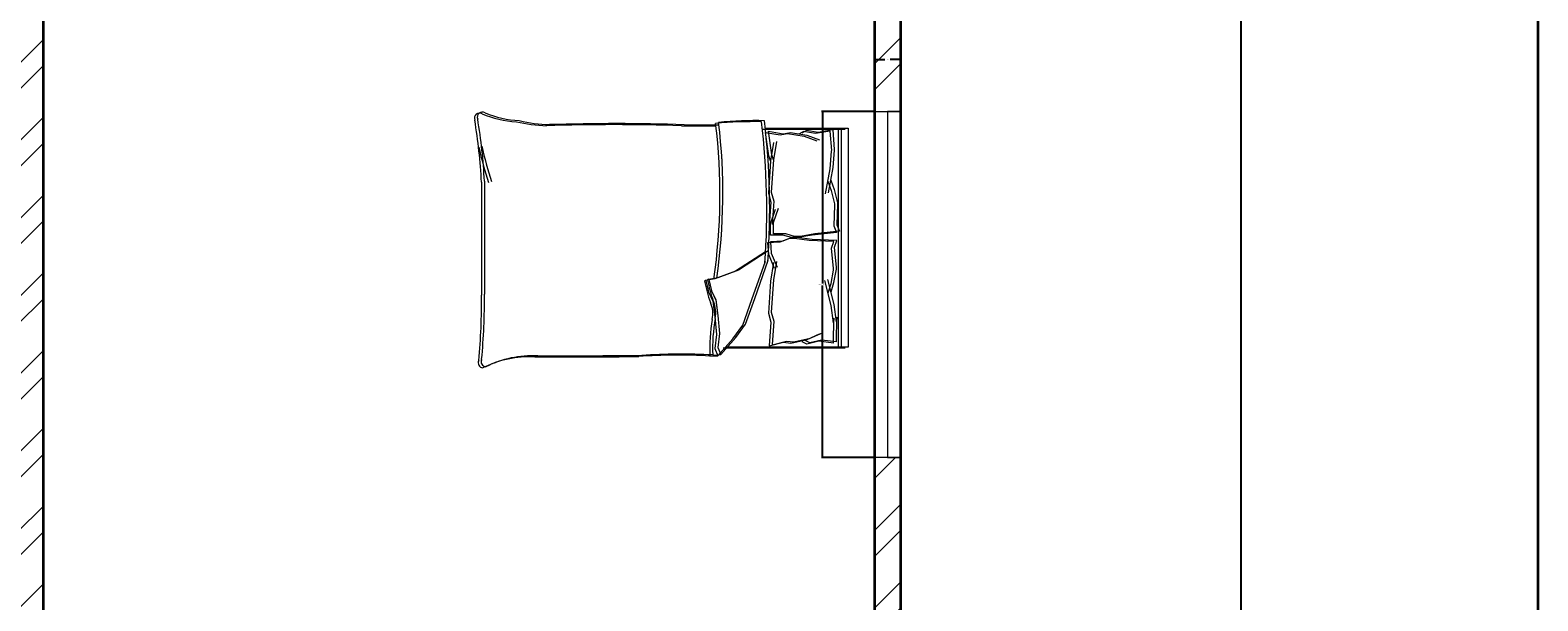
# Model space of a CAD drawing. Units: inches. Extents: x 1962 to 2771, y 1245 to 2660.
# Tile 113 of 114: x 2510 to 2771, y 2348 to 2447. Entities that reach past the tile are written whole.
import ezdxf

# ---------------------------------------------------------------- set-up
doc = ezdxf.new("R2010")
doc.units = ezdxf.units.IN
for name, color, linetype, lineweight in [('A-ANNO-DIMS', 2, 'Continuous', 18), ('A-ANNO-TTLB', 7, 'Continuous', 35), ('A-FURN', 8, 'Continuous', 13), ('A-GLAZ', 4, 'Continuous', 18), ('A-WALL', 7, 'Continuous', 35), ('A-WALL-PATT', 252, 'Continuous', 13)]:
    doc.layers.add(name, color=color, linetype=linetype, lineweight=lineweight)
doc.styles.get("Standard").update_dxf_attribs({"font": 'arial.ttf'})
doc.dimstyles.get("Standard").update_dxf_attribs({"dimtxt": 0.18, "dimasz": 0.18, "dimexe": 0.18, "dimexo": 0.0625, "dimgap": 0.09, "dimtad": 0, "dimtih": 1, "dimtoh": 1, "dimdec": 4, "dimzin": 0, "dimdsep": 46, "dimtxsty": 'Standard', "dimcen": 0.09, "dimadec": 0, "dimazin": 0, "dimtfac": 1, "dimtdec": 4, "dimtofl": 0, "dimtmove": 0, "dimatfit": 3, "dimfxl": 1, "dimtolj": 1, "dimtzin": 0, "dimarcsym": 0})

# ---------------------------------------------------------------- blocks, each defined once
blk = doc.blocks.new('BED-PLAN')
for p, q in [((22.05, 42.03), (19.47, 39.08)), ((22.05, 42.02), (19.47, 39.08)), ((22.56, 42.21), (19.98, 39.26)), ((22.56, 42.21), (19.98, 39.26)), ((23.44, 42.09), (22.05, 42.03, 3.08)), ((23.44, 42.09), (22.05, 42.02, 3.08)), ((22.55, 40.8), (22.05, 42.03)), ((22.55, 40.8), (22.05, 42.02)), ((23.95, 42.27), (22.56, 42.21, 3.08)), ((23.95, 42.27), (22.56, 42.21, 3.08)), ((23.06, 40.98), (22.56, 42.21)), ((23.06, 40.98), (22.56, 42.21)), ((0, 40.75), (21.15, 40.75)), ((0, 40.75), (21.15, 40.75)), ((0, 2.76), (0, 40.75)), ((0.51, 40.93), (21.66, 40.93)), ((0.51, 40.93), (21.66, 40.93)), ((1.22, 2.76), (1.22, 40.75)), ((1.22, 2.76), (1.22, 40.75)), ((1.73, 2.95), (1.73, 40.93)), ((1.73, 2.95), (1.73, 40.93)), ((2.03, 39.83), (1.96, 35.54)), ((2.03, 39.83), (1.96, 35.54)), ((2.03, 39.83), (4.58, 39.53)), ((2.03, 39.83), (4.58, 39.53)), ((2.54, 40.02), (2.46, 35.72)), ((2.54, 40.02), (2.46, 35.72)), ((2.54, 40.02), (5.09, 39.72)), ((2.54, 40.02), (5.09, 39.72)), ((6.56, 39.2), (4.43, 38.26)), ((6.56, 39.2), (4.43, 38.26)), ((4.58, 39.53), (6.63, 40.01)), ((4.58, 39.53), (6.63, 40.01)), ((7.07, 39.38), (4.94, 38.44)), ((7.07, 39.38), (4.94, 38.44)), ((5.09, 39.72), (7.14, 40.19)), ((5.09, 39.72), (7.14, 40.19)), ((9.4, 39.83), (6.56, 39.2)), ((9.4, 39.83), (6.56, 39.2)), ((6.63, 40.01), (7.46, 39.6)), ((6.63, 40.01), (7.46, 39.6)), ((9.91, 40.02), (7.07, 39.38)), ((9.91, 40.02), (7.07, 39.38)), ((7.14, 40.19), (7.97, 39.78)), ((7.14, 40.19), (7.97, 39.78)), ((10.68, 39.68), (9.4, 39.83)), ((10.68, 39.68), (9.4, 39.83)), ((11.19, 39.87), (9.91, 40.02)), ((11.19, 39.87), (9.91, 40.02)), ((13.17, 40.3), (10.68, 39.68)), ((13.17, 40.3), (10.68, 39.68)), ((13.68, 40.48), (11.19, 39.87)), ((13.68, 40.48), (11.19, 39.87)), ((12.85, 36.22), (13.17, 40.3)), ((12.85, 36.22), (13.17, 40.3)), ((13.36, 36.4), (13.68, 40.48)), ((13.36, 36.4), (13.68, 40.48)), ((19.98, 39.26), (18.26, 36.92)), ((19.98, 39.26), (18.26, 36.92)), ((22.3, 38.34), (22.55, 40.8)), ((22.3, 38.34), (22.55, 40.8)), ((22.81, 38.52), (23.06, 40.98)), ((22.81, 38.52), (23.06, 40.98)), ((17.75, 36.74), (16.15, 32.31)), ((17.75, 36.74), (16.15, 32.31)), ((18.26, 36.92), (16.66, 32.49)), ((18.26, 36.92), (16.66, 32.49)), ((19.47, 39.08), (17.75, 36.74)), ((19.47, 39.08), (17.75, 36.74)), ((22.55, 35.26), (22.3, 38.34)), ((22.55, 35.26), (22.3, 38.34)), ((23.06, 35.45), (22.81, 38.52)), ((23.06, 35.44), (22.81, 38.52)), ((1.96, 35.54), (2.02, 36.34)), ((1.96, 35.54), (2.02, 36.34)), ((2.02, 36.34), (2.44, 33.32)), ((2.02, 36.34), (2.44, 33.32)), ((2.46, 35.72), (2.53, 36.52)), ((2.46, 35.72), (2.53, 36.52)), ((2.53, 36.52), (2.95, 33.5)), ((2.53, 36.52), (2.95, 33.5)), ((13.3, 34.66), (12.85, 36.22)), ((13.3, 34.66), (12.85, 36.22)), ((12.95, 29.09), (13.3, 34.66)), ((12.95, 29.09), (13.3, 34.66)), ((13.8, 34.84), (13.36, 36.4)), ((13.8, 34.84), (13.36, 36.4)), ((13.46, 29.27), (13.8, 34.84)), ((13.46, 29.27), (13.8, 34.84)), ((22.92, 32.56), (22.55, 35.26)), ((22.92, 32.55), (22.55, 35.26)), ((23.42, 32.74), (23.06, 35.45)), ((23.42, 32.74), (23.06, 35.44)), ((2.44, 33.32), (3.52, 29.01)), ((2.44, 33.32), (3.52, 29.01)), ((2.95, 33.5), (4.02, 29.19)), ((2.95, 33.5), (4.02, 29.19)), ((3.43, 31.34), (2.96, 29.7)), ((3.43, 31.34), (2.96, 29.7)), ((16.15, 32.31), (13.82, 25.68)), ((16.15, 32.31), (13.82, 25.68)), ((16.66, 32.49), (14.33, 25.86)), ((16.66, 32.49), (14.33, 25.86)), ((23.65, 30.95), (22.92, 32.56)), ((23.65, 30.95), (22.92, 32.55)), ((24.16, 31.14), (23.42, 32.74)), ((24.16, 31.14), (23.42, 32.74)), ((62.99, 11.98), (62.99, 31.54)), ((62.99, 11.97), (62.99, 31.54)), ((63.5, 12.16), (63.5, 31.72)), ((63.5, 12.16), (63.5, 31.72)), ((2.45, 29.52), (2.02, 27.19)), ((2.45, 29.52), (2.02, 27.19)), ((2.92, 31.16), (2.45, 29.52)), ((2.92, 31.16), (2.45, 29.52)), ((2.96, 29.7), (2.52, 27.37)), ((2.96, 29.7), (2.52, 27.37)), ((12.42, 25.89), (12.95, 29.09)), ((12.42, 25.89), (12.95, 29.09)), ((12.93, 26.07), (13.46, 29.27)), ((12.93, 26.07), (13.46, 29.27)), ((18.98, 27.38), (22.55, 28.74)), ((18.98, 27.38), (22.55, 28.74)), ((19.49, 27.57), (23.06, 28.92)), ((19.49, 27.57), (23.06, 28.92)), ((22.55, 28.74), (24.15, 28.99)), ((22.55, 28.74), (24.15, 28.98)), ((23.06, 28.92), (24.65, 29.17)), ((23.06, 28.92), (24.65, 29.17)), ((24.15, 28.99), (23.65, 30.95)), ((24.15, 28.98), (23.65, 30.95)), ((24.65, 29.17), (24.16, 31.14)), ((24.65, 29.17), (24.16, 31.14)), ((2.02, 27.19), (2.03, 26.94)), ((2.02, 27.19), (2.03, 26.93)), ((2.03, 26.94), (2.37, 23.42)), ((2.03, 26.93), (2.37, 23.42)), ((2.52, 27.37), (2.54, 27.12)), ((2.52, 27.37), (2.54, 27.12)), ((2.54, 27.12), (2.88, 23.6)), ((2.54, 27.12), (2.88, 23.6)), ((13.31, 24.44), (12.28, 26.89)), ((13.31, 24.44), (12.28, 26.88)), ((13.81, 24.63), (12.79, 27.07)), ((13.81, 24.63), (12.79, 27.07)), ((13.82, 24.05), (18.98, 27.38)), ((13.82, 24.05), (18.98, 27.38)), ((14.33, 24.24), (19.49, 27.57)), ((14.33, 24.24), (19.49, 27.57)), ((2.88, 23.6), (2.49, 22.42)), ((2.88, 23.6), (2.49, 22.42)), ((13.43, 22.49), (13.31, 24.44)), ((13.43, 22.49), (13.31, 24.44)), ((13.94, 22.68), (13.81, 24.63)), ((13.94, 22.68), (13.81, 24.63)), ((1.49, 20.65), (5.74, 21.11)), ((1.49, 20.65), (5.74, 21.11)), ((2.37, 23.42), (1.98, 22.24)), ((2.37, 23.42), (1.98, 22.24)), ((1.98, 22.24), (6.25, 22.05)), ((1.98, 22.24), (6.25, 22.05)), ((1.99, 20.84), (6.25, 21.3)), ((1.99, 20.84), (6.25, 21.3)), ((2.49, 22.42), (6.76, 22.23)), ((2.49, 22.42), (6.76, 22.23)), ((5.74, 21.11), (8.27, 21.57)), ((5.74, 21.11), (8.27, 21.57)), ((6.25, 22.05), (8.81, 21.75)), ((6.25, 22.05), (8.81, 21.75)), ((6.25, 21.3), (8.78, 21.76)), ((6.25, 21.3), (8.78, 21.76)), ((6.76, 22.23), (9.31, 21.93)), ((6.76, 22.23), (9.31, 21.93)), ((8.27, 21.57), (9.3, 21.57)), ((8.27, 21.57), (9.3, 21.57)), ((8.78, 21.76), (9.81, 21.76)), ((8.78, 21.76), (9.81, 21.76)), ((8.81, 21.75), (9.84, 21.81)), ((8.81, 21.75), (9.84, 21.81)), ((9.3, 21.57), (10.8, 21.11)), ((9.3, 21.57), (10.8, 21.11)), ((9.31, 21.93), (10.35, 21.99)), ((9.31, 21.93), (10.35, 21.99)), ((9.81, 21.76), (11.3, 21.3)), ((9.81, 21.76), (11.3, 21.3)), ((9.84, 21.81), (11.3, 22.36)), ((9.84, 21.81), (11.3, 22.36)), ((10.35, 21.99), (11.81, 22.54)), ((10.35, 21.99), (11.81, 22.54)), ((10.8, 21.11), (12.93, 21.11)), ((10.8, 21.11), (12.93, 21.11)), ((11.3, 22.36), (13.43, 22.49)), ((11.3, 22.36), (13.43, 22.49)), ((11.3, 21.3), (13.44, 21.3)), ((11.3, 21.3), (13.44, 21.3)), ((11.81, 22.54), (13.94, 22.68)), ((11.81, 22.54), (13.94, 22.68)), ((12.93, 21.11), (12.93, 19.16)), ((12.93, 21.11), (12.93, 19.16)), ((13.44, 21.3), (13.44, 19.34)), ((13.44, 21.3), (13.44, 19.34)), ((1.95, 19.51), (1.49, 20.65)), ((1.95, 19.51), (1.49, 20.65)), ((1.83, 15.97), (1.95, 19.51)), ((1.83, 15.97), (1.95, 19.51)), ((2.45, 19.69), (1.99, 20.84)), ((2.45, 19.69), (1.99, 20.84)), ((2.34, 16.15), (2.45, 19.69)), ((2.34, 16.15), (2.45, 19.69)), ((12.93, 19.16), (12.06, 16.66)), ((12.93, 19.16), (12.06, 16.66)), ((13.44, 19.34), (12.57, 16.84)), ((13.44, 19.34), (12.57, 16.84)), ((12.85, 15.41), (13.17, 19.49)), ((12.85, 15.41), (13.17, 19.49)), ((13.36, 15.59), (13.68, 19.67)), ((13.36, 15.59), (13.68, 19.67)), ((1.83, 15.72), (1.83, 15.97)), ((1.83, 15.72), (1.83, 15.97)), ((2.41, 13.42), (1.83, 15.72)), ((2.41, 13.42), (1.83, 15.72)), ((2.34, 15.9), (2.34, 16.15)), ((2.34, 15.9), (2.34, 16.15)), ((2.91, 13.6), (2.34, 15.9)), ((2.91, 13.6), (2.34, 15.9)), ((2.98, 11.81), (2.41, 13.42)), ((2.98, 11.81), (2.41, 13.42)), ((2.64, 9.63), (3.44, 13.99)), ((2.64, 9.63), (3.44, 13.99)), ((3.49, 11.99), (2.91, 13.6)), ((3.49, 11.99), (2.91, 13.6)), ((3.14, 9.81), (3.95, 14.17)), ((3.14, 9.81), (3.95, 14.17)), ((13.3, 13.85), (12.85, 15.41)), ((13.3, 13.85), (12.85, 15.41)), ((12.95, 8.28), (13.3, 13.85)), ((12.95, 8.28), (13.3, 13.85)), ((13.8, 14.03), (13.36, 15.59)), ((13.8, 14.03), (13.36, 15.59)), ((13.46, 8.46), (13.8, 14.03)), ((13.46, 8.46), (13.8, 14.03)), ((2.41, 6.59), (2.64, 9.63)), ((2.41, 6.59), (2.64, 9.63)), ((2.91, 6.77), (3.14, 9.81)), ((2.91, 6.77), (3.14, 9.81)), ((12.42, 5.07), (12.95, 8.28)), ((12.42, 5.07), (12.95, 8.28)), ((12.93, 5.26), (13.46, 8.46)), ((12.93, 5.26), (13.46, 8.46)), ((12.95, 8.28), (13.21, 7.38)), ((12.95, 8.28), (13.21, 7.38)), ((13.46, 8.46), (13.72, 7.56)), ((13.46, 8.46), (13.72, 7.56)), ((2.39, 6.5), (2.41, 6.59)), ((2.39, 6.5), (2.41, 6.59)), ((2.65, 3.1), (2.39, 6.5)), ((2.65, 3.1), (2.39, 6.5)), ((2.9, 6.68), (2.91, 6.77)), ((2.9, 6.68), (2.91, 6.77)), ((3.16, 3.28), (2.9, 6.68)), ((3.16, 3.28), (2.9, 6.68)), ((13.21, 7.38), (13.78, 3.33)), ((13.21, 7.38), (13.78, 3.33)), ((13.72, 7.56), (14.29, 3.51)), ((13.72, 7.56), (14.29, 3.51)), ((14.4, 2.76), (0, 2.76)), ((14.4, 2.76), (0, 2.76)), ((14.9, 2.95), (0.51, 2.95)), ((14.9, 2.95), (0.51, 2.95)), ((2.64, 3.1), (5.16, 3.56)), ((2.64, 3.1), (5.16, 3.56)), ((3.14, 3.28), (5.67, 3.74)), ((3.14, 3.28), (5.67, 3.74)), ((7.12, 4.02), (4.93, 4.82)), ((7.12, 4.02), (4.93, 4.82)), ((5.16, 3.56), (7.23, 3.21)), ((5.16, 3.56), (7.23, 3.21)), ((7.63, 4.2), (5.44, 5)), ((7.63, 4.2), (5.44, 5)), ((5.67, 3.74), (7.74, 3.39)), ((5.67, 3.74), (7.74, 3.39)), ((9.99, 3.56), (7.12, 4.02)), ((9.99, 3.56), (7.12, 4.02)), ((7.23, 3.21), (8.04, 3.67)), ((7.23, 3.21), (8.04, 3.67)), ((10.5, 3.74), (7.63, 4.2)), ((10.5, 3.74), (7.63, 4.2)), ((7.74, 3.39), (8.55, 3.85)), ((7.74, 3.39), (8.55, 3.85)), ((11.26, 3.79), (9.99, 3.56)), ((11.26, 3.79), (9.99, 3.56)), ((11.76, 3.97), (10.5, 3.74)), ((11.76, 3.97), (10.5, 3.74)), ((13.78, 3.33), (11.26, 3.79)), ((13.78, 3.33), (11.26, 3.79)), ((14.29, 3.51), (11.76, 3.97)), ((14.29, 3.51), (11.76, 3.97))]:
    blk.add_line(p, q)
for centre, radius, start, end in [((-5.29, 40.8), 28.76, 349.8763, 2.5657), ((-5.29, 40.8), 28.76, 349.8763, 2.5657), ((28.87, 144.88), 102.94, 266.9791, 273.8365), ((28.87, 144.88), 102.94, 266.9791, 273.8365), ((-4.78, 40.98), 28.76, 349.8763, 2.5657), ((-4.78, 40.98), 28.76, 349.8763, 2.5657), ((29.37, 145.06), 102.94, 266.9791, 273.8365), ((29.37, 145.06), 102.94, 266.9791, 273.8365), ((53.91, -3583.94), 3626.16, 90.00217, 90.28689), ((53.91, -3583.94), 3626.16, 90.00217, 90.28689), ((54.42, -3583.75), 3626.16, 90.00217, 90.28689), ((54.42, -3583.75), 3626.16, 90.00217, 90.28689), ((54.58, 60.54), 18.33, 267.4714, 296.4681), ((54.58, 60.54), 18.33, 267.4714, 296.4681), ((55.09, 60.72), 18.33, 267.4714, 296.4681), ((55.09, 60.72), 18.33, 267.4714, 296.4681), ((62.69, 43.25), 0.876, 332.6588, 86.02), ((62.69, 43.25), 0.876, 332.6588, 86.02), ((168.74, 32.71), 105.75, 174.4998, 180.6351), ((168.74, 32.71), 105.75, 174.4998, 180.6351), ((63.2, 43.43), 0.876, 332.6588, 86.02), ((63.2, 43.43), 0.876, 332.6588, 86.02), ((169.24, 32.89), 105.75, 174.4998, 180.6351), ((169.24, 32.89), 105.75, 174.4998, 180.6351), ((27.87, 34.77), 4.95, 168.6608, 203.7384), ((27.87, 34.77), 4.95, 168.6608, 203.7384), ((28.38, 34.95), 4.95, 168.6608, 203.7384), ((28.38, 34.95), 4.95, 168.6608, 203.7384), ((1.18, 24.77), 23.57, 10.6617, 19.8806), ((1.18, 24.76), 23.57, 10.6617, 19.8806), ((1.69, 24.95), 23.57, 10.6617, 19.8806), ((1.69, 24.95), 23.57, 10.6617, 19.8806), ((124.25, 14.12), 102.56, 171.7845, 186.9006), ((124.25, 14.11), 102.56, 171.7845, 186.9006), ((124.76, 14.3), 102.56, 171.7845, 186.9006), ((124.76, 14.3), 102.56, 171.7845, 186.9006), ((24.2, 29.12), 0.147, 250.2464, 1.1377), ((24.2, 29.12), 0.147, 250.2464, 1.1377), ((24.7, 29.3), 0.147, 250.2464, 1.1377), ((24.7, 29.3), 0.147, 250.2464, 1.1377), ((144.71, 16.98), 131.13, 176.0865, 186.7821), ((144.71, 16.98), 131.13, 176.0865, 186.7821), ((145.22, 17.16), 131.13, 176.0865, 186.7821), ((145.22, 17.16), 131.13, 176.0865, 186.7821), ((-18.85, -13.69), 84.62, 13.3832, 17.7053), ((-18.85, -13.69), 84.62, 13.3832, 17.7053), ((-18.34, -13.51), 84.62, 13.3832, 17.7053), ((-18.34, -13.51), 84.62, 13.3832, 17.7053), ((159.64, 17.03), 96.78, 182.9958, 189.4091), ((159.64, 17.03), 96.78, 182.9958, 189.4091), ((160.15, 17.21), 96.78, 182.9958, 189.4091), ((160.15, 17.21), 96.78, 182.9958, 189.4091), ((15.97, 67.7), 66.22, 268.7218, 275.604), ((15.97, 67.7), 66.22, 268.7218, 275.604), ((16.48, 67.88), 66.22, 268.7218, 275.604), ((16.48, 67.88), 66.22, 268.7218, 275.604), ((24.78, -132.99), 135.22, 88.4762, 91.0082), ((24.78, -132.99), 135.22, 88.4762, 91.0082), ((25.29, -132.81), 135.22, 88.4762, 91.0082), ((25.29, -132.81), 135.22, 88.4762, 91.0082), ((40.23, 385.38), 383.38, 268.2277, 271.7185), ((40.23, 385.38), 383.38, 268.2277, 271.7185), ((40.74, 385.56), 383.38, 268.2277, 271.7185), ((40.74, 385.56), 383.38, 268.2277, 271.7185), ((51.28, -21.38), 23.56, 76.0648, 88.9113), ((51.28, -21.38), 23.56, 76.0648, 88.9113), ((51.79, -21.2), 23.56, 76.0648, 88.9113), ((51.79, -21.2), 23.56, 76.0648, 88.9113), ((55.86, -17.22), 18.73, 67.9751, 86.652), ((55.86, -17.22), 18.73, 67.9751, 86.652), ((56.37, -17.03), 18.73, 67.9751, 86.652), ((56.37, -17.03), 18.73, 67.9751, 86.652), ((63.37, 0.87), 0.866, 236.1736, 23.4781), ((63.37, 0.87), 0.866, 236.1736, 23.4781), ((63.87, 1.05), 0.866, 236.1736, 23.4781), ((63.87, 1.05), 0.866, 236.1736, 23.4781)]:
    blk.add_arc(centre, radius, start, end)
blk = doc.blocks.new('WIN-60IN-B')
for p, q in [((0, 60), (4.5, 60)), ((4.5, 60), (2.25, 60)), ((2.25, 60), (2.25, 0)), ((4.5, 0), (0, 0)), ((2.25, 0), (4.5, 0))]:
    blk.add_line(p, q)
blk = doc.blocks.new('*D24')
at = {"layer": 'A-ANNO-DIMS', "color": 0, "lineweight": -2, "transparency": 16777216}
for p, q in [((2656.24, 2432.57), (2647.13, 2432.57)), ((2647.31, 2432.39), (2647.31, 2402.75)), ((2647.31, 2372.75), (2647.31, 2402.39)), ((2656.24, 2372.57), (2647.13, 2372.57))]:
    blk.add_line(p, q, dxfattribs=at)
at = {"layer": 'A-ANNO-DIMS', "color": 0, "transparency": 16777216}
for points in [[(2647.28, 2432.39), (2647.34, 2432.39), (2647.31, 2432.57)], [(2647.28, 2372.75), (2647.34, 2372.75), (2647.31, 2372.57)]]:
    blk.add_solid(points, dxfattribs=at)
at = {"layer": 'Defpoints', "color": 0, "transparency": 16777216}
for p in [(2647.31, 2432.57), (2656.31, 2432.57), (2656.31, 2372.57)]:
    blk.add_point(p, dxfattribs=at)
at = {"layer": 'A-ANNO-DIMS', "color": 0, "transparency": 16777216, "insert": (2647.31, 2402.57), "char_height": 0.18, "attachment_point": 5}
blk.add_mtext('\\A1;W3B 60 TYP.', dxfattribs=at)
blk = doc.blocks.new('*D25')
at = {"layer": 'A-ANNO-DIMS', "color": 0, "lineweight": -2, "transparency": 16777216}
for p, q in [((2656.31, 2432.63), (2656.31, 2441.75)), ((2656.49, 2441.57), (2658.1, 2441.57)), ((2660.63, 2441.57), (2659.02, 2441.57)), ((2660.81, 2432.63), (2660.81, 2441.75))]:
    blk.add_line(p, q, dxfattribs=at)
at = {"layer": 'A-ANNO-DIMS', "color": 0, "transparency": 16777216}
for points in [[(2656.49, 2441.6), (2656.49, 2441.54), (2656.31, 2441.57)], [(2660.63, 2441.6), (2660.63, 2441.54), (2660.81, 2441.57)]]:
    blk.add_solid(points, dxfattribs=at)
at = {"layer": 'Defpoints', "color": 0, "transparency": 16777216}
for p in [(2660.81, 2441.57), (2656.31, 2432.57), (2660.81, 2432.57)]:
    blk.add_point(p, dxfattribs=at)
at = {"layer": 'A-ANNO-DIMS', "color": 0, "transparency": 16777216, "insert": (2658.56, 2441.57), "char_height": 0.18, "attachment_point": 5}
blk.add_mtext('\\A1;5 TYP.', dxfattribs=at)
blk = doc.blocks.new('*D40')
at = {"layer": 'A-ANNO-DIMS', "color": 0, "lineweight": -2, "transparency": 16777216}
for p, q in [((2072.02, 2033.91), (2072.02, 2583.47)), ((2072.2, 2583.29), (2366.02, 2583.29)), ((2660.63, 2583.29), (2366.81, 2583.29)), ((2660.81, 2524.41), (2660.81, 2583.47))]:
    blk.add_line(p, q, dxfattribs=at)
at = {"layer": 'A-ANNO-DIMS', "color": 0, "transparency": 16777216}
for points in [[(2072.2, 2583.32), (2072.2, 2583.26), (2072.02, 2583.29)], [(2660.63, 2583.32), (2660.63, 2583.26), (2660.81, 2583.29)]]:
    blk.add_solid(points, dxfattribs=at)
at = {"layer": 'Defpoints', "color": 0, "transparency": 16777216}
for p in [(2660.81, 2583.29), (2660.81, 2524.34), (2072.02, 2033.84)]:
    blk.add_point(p, dxfattribs=at)
at = {"layer": 'A-ANNO-DIMS', "color": 0, "transparency": 16777216, "insert": (2366.41, 2583.29), "char_height": 0.18, "attachment_point": 5}
blk.add_mtext('\\A1;588.8', dxfattribs=at)
blk = doc.blocks.new('*D42')
at = {"layer": 'A-ANNO-DIMS', "color": 0, "lineweight": -2, "transparency": 16777216}
for p, q in [((2660.87, 2524.34), (2719.94, 2524.34)), ((2719.76, 2524.16), (2719.76, 1979.28)), ((2719.76, 1434.02), (2719.76, 1978.91)), ((2660.87, 1433.84), (2719.94, 1433.84))]:
    blk.add_line(p, q, dxfattribs=at)
at = {"layer": 'A-ANNO-DIMS', "color": 0, "transparency": 16777216}
for points in [[(2719.73, 2524.16), (2719.79, 2524.16), (2719.76, 2524.34)], [(2719.73, 1434.02), (2719.79, 1434.02), (2719.76, 1433.84)]]:
    blk.add_solid(points, dxfattribs=at)
at = {"layer": 'Defpoints', "color": 0, "transparency": 16777216}
for p in [(2660.81, 2524.34), (2719.76, 2524.34), (2660.81, 1433.84)]:
    blk.add_point(p, dxfattribs=at)
at = {"layer": 'A-ANNO-DIMS', "color": 0, "transparency": 16777216, "insert": (2719.76, 1979.09), "char_height": 0.18, "attachment_point": 5}
blk.add_mtext('\\A1;1090.5', dxfattribs=at)

msp = doc.modelspace()

# ---------------------------------------------------------------- hatches: boundary and pattern name
at = {"layer": 'A-WALL-PATT'}
h = msp.add_hatch(dxfattribs=at)
h.set_pattern_fill('ANSI32', color=256)
h.paths.add_polyline_path([(2090.8074, 2467.3437), (2141.6481, 2467.3437), (2141.6481, 2469.5937), (2141.6481, 2471.8437), (2086.3074, 2471.8437), (2086.3074, 2422.5333), (2090.8074, 2422.5333)])
h.paths.add_polyline_path([(2282.7664, 2471.8437), (2204.8982, 2471.8437), (2204.8982, 2467.3437), (2234.8074, 2467.3437), (2234.8074, 2311.3437), (2228.7492, 2311.3437), (2228.7492, 2306.8437), (2234.8074, 2306.8437), (2331.9227, 2306.8437), (2331.9227, 2309.0937), (2331.9227, 2311.3437), (2239.3074, 2311.3437), (2239.3074, 2467.3437), (2282.7664, 2467.3437), (2282.7664, 2469.5937)])
h.paths.add_polyline_path([(2471.4531, 2519.8437), (2552.011, 2519.8437), (2564.3996, 2519.8437), (2564.3996, 2511.1389), (2568.8996, 2511.1389), (2568.8996, 2524.3437), (2466.9531, 2524.3437), (2466.9531, 2471.8437), (2450.0749, 2471.8437), (2446.4672, 2471.8437), (2446.4672, 2467.3437), (2450.0749, 2467.3437), (2475.9988, 2467.3437), (2475.9988, 2469.5937), (2475.9988, 2471.8437), (2471.4531, 2471.8437)])
h.paths.add_polyline_path([(2575.2231, 2469.5937), (2575.2231, 2471.8437), (2568.8996, 2471.8437), (2568.8996, 2487.1389), (2564.3996, 2487.1389), (2564.3996, 2471.8437), (2556.511, 2471.8437), (2499.2904, 2471.8437), (2499.2904, 2467.3437), (2507.8074, 2467.3437), (2507.8074, 2311.3437), (2414.863, 2311.3437), (2414.863, 2306.8437), (2512.3074, 2306.8437), (2517.0114, 2306.8437), (2517.0114, 2309.0937), (2517.0114, 2311.3437), (2512.3074, 2311.3437), (2512.3074, 2467.3437), (2575.2231, 2467.3437)])
h.paths.add_polyline_path([(2660.8074, 2471.8437), (2600.9602, 2471.8437), (2600.9602, 2467.3437), (2656.3074, 2467.3437), (2656.3074, 2432.5704), (2660.8074, 2432.5704)])
h.paths.add_polyline_path([(2660.8074, 2372.5704), (2656.3074, 2372.5704), (2656.3074, 2311.3437), (2600.276, 2311.3437), (2600.276, 2309.0937), (2600.276, 2306.8437), (2656.3074, 2306.8437), (2656.3074, 2296.2593), (2660.8074, 2296.2593)])
h.paths.add_polyline_path([(2572.3074, 2306.8437), (2577.1385, 2306.8437), (2577.1385, 2311.3437), (2551.082, 2311.3437), (2551.082, 2306.8437), (2567.8074, 2306.8437), (2567.8074, 2258.8437), (2540.0574, 2258.8437), (2540.0574, 2256.5937), (2540.0574, 2254.3437), (2567.8074, 2254.3437), (2656.3074, 2254.3437), (2656.3074, 2236.9085), (2660.8074, 2236.9085), (2660.8074, 2272.2593), (2656.3074, 2272.2593), (2656.3074, 2258.8437), (2572.3074, 2258.8437)])
h.paths.add_polyline_path([(2512.3074, 2254.3437), (2518.8716, 2254.3437), (2518.8716, 2256.5937), (2518.8716, 2258.8437), (2507.8074, 2258.8437), (2507.8074, 2177.8437), (2567.8074, 2177.8437), (2567.8074, 2172.9628), (2572.3074, 2172.9628), (2572.3074, 2177.8437), (2656.3074, 2177.8437), (2656.3074, 2166.4846), (2660.8074, 2166.4846), (2660.8074, 2200.9085), (2656.3074, 2200.9085), (2656.3074, 2182.3437), (2512.3074, 2182.3437)])
h.paths.add_polyline_path([(2656.3074, 2129.8437), (2572.3074, 2129.8437), (2572.3074, 2150.3044), (2570.0574, 2150.3044), (2567.8074, 2150.3044), (2567.8074, 2129.8437), (2507.8074, 2129.8437), (2507.8074, 2116.3027), (2510.0574, 2116.3027), (2512.3074, 2116.3027), (2512.3074, 2125.3437), (2567.8074, 2125.3437), (2572.3074, 2125.3437), (2656.3074, 2125.3437)])
h.paths.add_polyline_path([(2090.8074, 2362.5333), (2086.3074, 2362.5333), (2086.3074, 2298.6242), (2090.8074, 2298.6242), (2090.8074, 2306.8437), (2174.8074, 2306.8437), (2174.8074, 2286.4178), (2179.3074, 2286.4178), (2179.3074, 2306.8437), (2192.8641, 2306.8437), (2192.8641, 2309.0937), (2192.8641, 2311.3437), (2090.8074, 2311.3437)])
h.paths.add_polyline_path([(2209.156, 2258.8437), (2179.3074, 2258.8437), (2179.3074, 2263.2236), (2177.0574, 2263.2236), (2174.8074, 2263.2236), (2174.8074, 2258.8437), (2090.8074, 2258.8437), (2090.8074, 2274.6242), (2086.3074, 2274.6242), (2086.3074, 2238.2967), (2088.5574, 2238.2967), (2090.8074, 2238.2967), (2090.8074, 2254.3437), (2209.156, 2254.3437)])
h.paths.add_polyline_path([(2090.8074, 2177.8437), (2234.8074, 2177.8437), (2234.8074, 2173.1428), (2239.3074, 2173.1428), (2239.3074, 2258.8437), (2230.8442, 2258.8437), (2230.8442, 2256.5937), (2230.8442, 2254.3437), (2234.8074, 2254.3437), (2234.8074, 2182.3437), (2090.8074, 2182.3437), (2090.8074, 2202.2967), (2086.3074, 2202.2967), (2086.3074, 2140.0389), (2090.8074, 2140.0389)])
h.paths.add_polyline_path([(2090.8074, 2080.0389), (2086.3074, 2080.0389), (2086.3074, 2033.8437), (2090.8074, 2033.8437)], flags=17)
h.paths.add_polyline_path([(2244.9405, 2033.8437), (2239.3074, 2033.8437), (2239.3074, 2142.0665), (2237.2592, 2142.0665), (2234.8074, 2142.0665), (2234.8074, 2033.8437), (2090.8074, 2033.8437), (2076.5204, 2033.8437), (2072.0204, 2033.8437), (2072.0204, 2000.4493), (2076.5204, 2000.4493), (2076.5204, 2029.3437), (2090.8074, 2029.3437), (2244.9405, 2029.3437), (2244.9405, 2031.5937)])
h.paths.add_polyline_path([(2234.8074, 1933.3437), (2076.5204, 1933.3437), (2076.5204, 1952.4493), (2074.2704, 1952.4493), (2072.0204, 1952.4493), (2072.0204, 1933.3437), (2072.0204, 1928.8437), (2234.8074, 1928.8437)])
h.paths.add_polyline_path([(2090.8074, 1928.8437), (2086.3074, 1928.8437), (2086.3074, 1906.5013), (2090.8074, 1906.5013)])
h.paths.add_polyline_path([(2090.8074, 1846.5013), (2086.3074, 1846.5013), (2086.3074, 1769.9917), (2088.5574, 1769.9917), (2090.8074, 1769.9917), (2090.8074, 1780.3437), (2234.8074, 1780.3437), (2234.8074, 1708.3437), (2230.3764, 1708.3437), (2230.3764, 1703.8437), (2239.3074, 1703.8437), (2239.3074, 1792.6669), (2237.0574, 1792.6669), (2234.8074, 1792.6669), (2234.8074, 1784.8437), (2090.8074, 1784.8437)])
h.paths.add_polyline_path([(2239.3074, 1928.8437), (2244.9405, 1928.8437), (2244.9405, 1931.0937), (2244.9405, 1933.3437), (2234.8074, 1933.3437), (2234.8074, 1928.8437), (2234.8074, 1825.5949), (2239.3074, 1825.5949)])
h.paths.add_polyline_path([(2148.0425, 1649.0937), (2148.0425, 1651.3437), (2090.8074, 1651.3437), (2090.8074, 1646.8437), (2148.0425, 1646.8437)], flags=0)
h.paths.add_polyline_path([(2207.5601, 1708.3437), (2090.8074, 1708.3437), (2090.8074, 1703.8437), (2174.8074, 1703.8437), (2174.8074, 1651.3437), (2170.4457, 1651.3437), (2170.4457, 1646.8437), (2195.9924, 1646.8437), (2195.9924, 1649.0937), (2195.9924, 1651.3437), (2179.3074, 1651.3437), (2179.3074, 1703.8437), (2207.5601, 1703.8437), (2207.5601, 1706.0937)])
h.paths.add_polyline_path([(2090.8074, 1733.9917), (2086.3074, 1733.9917), (2086.3074, 1696.1032), (2088.5574, 1696.1032), (2090.8074, 1696.1032)])
h.paths.add_polyline_path([(2090.8074, 1672.1032), (2086.3074, 1672.1032), (2086.3074, 1600.3335), (2090.8074, 1600.3335)])
h.paths.add_polyline_path([(2090.8074, 1540.3335), (2086.3074, 1540.3335), (2086.3074, 1486.3437), (2139.6766, 1486.3437), (2139.6766, 1490.8437), (2090.8074, 1490.8437)])
h.paths.add_polyline_path([(2302.3876, 1490.8437), (2239.3074, 1490.8437), (2239.3074, 1646.8437), (2335.9994, 1646.8437), (2335.9994, 1651.3437), (2229.884, 1651.3437), (2229.884, 1646.8437), (2234.8074, 1646.8437), (2234.8074, 1490.8437), (2202.7103, 1490.8437), (2202.7103, 1488.5937), (2202.7103, 1486.3437), (2275.0699, 1486.3437), (2275.0699, 1475.772), (2279.5699, 1475.772), (2279.5699, 1486.3437), (2302.3876, 1486.3437)])
h.paths.add_polyline_path([(2279.5699, 1451.772), (2275.0699, 1451.772), (2275.0699, 1438.3437), (2174.8074, 1438.3437), (2174.8074, 1486.3437), (2179.7922, 1486.3437), (2179.7922, 1490.8437), (2163.3585, 1490.8437), (2163.3585, 1488.5937), (2163.3585, 1486.3437), (2170.3074, 1486.3437), (2170.3074, 1433.8437), (2279.5699, 1433.8437)])
h.paths.add_polyline_path([(2427.2363, 1490.8437), (2375.8074, 1490.8437), (2375.8074, 1646.8437), (2381.6401, 1646.8437), (2381.6401, 1651.3437), (2365.887, 1651.3437), (2365.887, 1649.0937), (2365.887, 1646.8437), (2371.3074, 1646.8437), (2371.3074, 1490.8437), (2327.5627, 1490.8437), (2327.5627, 1488.5937), (2327.5627, 1486.3437), (2371.3074, 1486.3437), (2371.3074, 1433.8437), (2375.8074, 1433.8437), (2375.8074, 1486.3437), (2427.2363, 1486.3437)])
h.paths.add_polyline_path([(2512.3074, 1646.8437), (2519.4351, 1646.8437), (2519.4351, 1649.0937), (2519.4351, 1651.3437), (2507.8074, 1651.3437), (2416.0063, 1651.3437), (2416.0063, 1649.0937), (2416.0063, 1646.8437), (2507.8074, 1646.8437), (2507.8074, 1490.8437), (2497.0532, 1490.8437), (2497.0532, 1488.5937), (2497.0532, 1486.3437), (2574.9344, 1486.3437), (2574.9344, 1476.0181), (2579.4344, 1476.0181), (2579.4344, 1486.3437), (2584.4872, 1486.3437), (2584.3074, 1490.8437), (2512.3074, 1490.8437)])
h.paths.add_polyline_path([(2470.5091, 1486.3437), (2473.9767, 1486.3437), (2473.9767, 1490.8437), (2449.6605, 1490.8437), (2449.6605, 1488.5937), (2449.6605, 1486.3437), (2466.0091, 1486.3437), (2466.0091, 1433.8437), (2470.5091, 1433.8437), (2579.4344, 1433.8437), (2579.4344, 1452.0181), (2574.9344, 1452.0181), (2574.9344, 1438.3437), (2554.5091, 1438.3437), (2470.5091, 1438.3437)])
h.paths.add_polyline_path([(2656.3074, 1490.8437), (2611.86, 1490.8437), (2611.86, 1486.3437), (2656.3074, 1486.3437)])
h.paths.add_polyline_path([(2660.8074, 1532.7007), (2658.5574, 1532.7007), (2656.3074, 1532.7007), (2656.3074, 1486.3437), (2660.8074, 1486.3437)])
h.paths.add_polyline_path([(2660.8074, 1664.9663), (2656.3074, 1664.9663), (2656.3074, 1651.3437), (2602.2313, 1651.3437), (2602.2313, 1646.8437), (2656.3074, 1646.8437), (2656.3074, 1592.7007), (2660.8074, 1592.7007)])
h.paths.add_polyline_path([(2660.8074, 1724.5221), (2656.3074, 1724.5221), (2656.3074, 1703.8437), (2542.4725, 1703.8437), (2542.4725, 1699.3437), (2567.8074, 1699.3437), (2567.8074, 1651.3437), (2552.7766, 1651.3437), (2552.7766, 1649.0937), (2552.7766, 1646.8437), (2577.2878, 1646.8437), (2577.2878, 1649.0937), (2577.2878, 1651.3437), (2572.3074, 1651.3437), (2572.3074, 1699.3437), (2656.3074, 1699.3437), (2656.3074, 1688.9663), (2660.8074, 1688.9663)])
h.paths.add_polyline_path([(2660.8074, 1880.6524), (2656.3074, 1880.6524), (2656.3074, 1832.8437), (2512.3074, 1832.8437), (2512.3074, 1837.8959), (2507.8074, 1837.8959), (2507.8074, 1828.3437), (2567.8074, 1828.3437), (2567.8074, 1804.3437), (2572.3074, 1804.3437), (2572.3074, 1828.3437), (2656.3074, 1828.3437), (2656.3074, 1818.6778), (2660.8074, 1818.6778)])
h.paths.add_polyline_path([(2660.8074, 1794.6778), (2656.3074, 1794.6778), (2656.3074, 1780.3437), (2572.3074, 1780.3437), (2572.3074, 1783.0303), (2570.0574, 1783.0303), (2567.8074, 1783.0303), (2567.8074, 1780.3437), (2507.8074, 1780.3437), (2507.8074, 1699.3437), (2517.8858, 1699.3437), (2517.8858, 1701.5937), (2517.8858, 1703.8437), (2512.3074, 1703.8437), (2512.3074, 1775.8437), (2656.3074, 1775.8437), (2656.3074, 1760.5221), (2660.8074, 1760.5221)])
h.paths.add_polyline_path([(2660.8074, 1981.3437), (2660.8074, 2020.2808), (2658.5574, 2020.2808), (2656.3074, 2020.2808), (2656.3074, 1981.3437), (2512.3074, 1981.3437), (2512.3074, 2086.6996), (2507.8074, 2086.6996), (2507.8074, 1981.3437), (2375.8074, 1981.3437), (2375.8074, 1986.8505), (2373.5574, 1986.8505), (2371.3074, 1986.8505), (2371.3074, 1973.2607), (2375.8074, 1973.2607), (2375.8074, 1976.8437), (2507.8074, 1976.8437), (2507.8074, 1865.4281), (2510.0574, 1865.4281), (2512.3074, 1865.4281), (2512.3074, 1976.8437), (2660.8074, 1976.8437)])
h.paths.add_polyline_path([(2375.8074, 1940.297), (2373.5574, 1940.297), (2371.3074, 1940.297), (2371.3074, 1933.3437), (2278.4434, 1933.3437), (2278.4434, 1928.8437), (2371.3074, 1928.8437), (2371.3074, 1651.3437), (2375.8074, 1651.3437)])
h.paths.add_polyline_path([(2660.8074, 1976.8437), (2656.3074, 1976.8437), (2656.3074, 1940.6524), (2660.8074, 1940.6524)], flags=17)
h.paths.add_polyline_path([(2660.8074, 2142.4846), (2656.3074, 2142.4846), (2656.3074, 2080.2808), (2660.8074, 2080.2808)])
h.paths.add_polyline_path([(2381.4189, 2311.3437), (2375.8074, 2311.3437), (2375.8074, 2467.3437), (2424.7242, 2467.3437), (2424.7242, 2469.5937), (2424.7242, 2471.8437), (2375.8074, 2471.8437), (2375.8074, 2524.3437), (2371.3074, 2524.3437), (2371.3074, 2471.8437), (2307.2097, 2471.8437), (2307.2097, 2467.3437), (2371.3074, 2467.3437), (2371.3074, 2311.3437), (2366.8901, 2311.3437), (2366.8901, 2306.8437), (2371.3074, 2306.8437), (2371.3074, 2033.8437), (2279.6589, 2033.8437), (2279.6589, 2029.3437), (2371.3074, 2029.3437), (2371.3074, 2014.2598), (2375.8074, 2014.2598), (2375.8074, 2306.8437), (2381.4189, 2306.8437)])
h.paths.add_polyline_path([(2263.3074, 2524.3437), (2170.3074, 2524.3437), (2170.3074, 2519.8437), (2170.3074, 2471.8437), (2165.0312, 2471.8437), (2165.0312, 2467.3437), (2179.6721, 2467.3437), (2179.6721, 2469.5161), (2179.6721, 2471.8437), (2174.8074, 2471.8437), (2174.8074, 2519.8437), (2258.8074, 2519.8437), (2258.8074, 2511.6436), (2263.3074, 2511.6436)])
h.paths.add_polyline_path([(2245.0232, 1361.4123), (2492.9468, 1361.4123), (2492.9468, 1398.505), (2245.0232, 1398.505)], flags=9)
h.paths.add_polyline_path([(2388.1434, 2086.6936), (2425.0704, 2086.6936), (2425.0704, 2105.3509), (2388.1434, 2105.3509)], flags=9)
h.paths.add_polyline_path([(2404.922, 2242.6744), (2445.7337, 2242.6744), (2445.7337, 2261.3318), (2404.922, 2261.3318)], flags=9)
h.paths.add_polyline_path([(2269.4107, 2156.7935), (2306.3378, 2156.7935), (2306.3378, 2175.4508), (2269.4107, 2175.4508)], flags=9)
h.paths.add_polyline_path([(2269.3277, 2233.4343), (2306.2547, 2233.4343), (2306.2547, 2252.0917), (2269.3277, 2252.0917)], flags=9)
h.paths.add_polyline_path([(2431.6052, 2320.6922), (2470.4456, 2320.6922), (2470.4456, 2339.3495), (2431.6052, 2339.3495)], flags=25)
h.paths.add_polyline_path([(2249.6902, 2315.7608), (2288.5306, 2315.7608), (2288.5306, 2334.4182), (2249.6902, 2334.4182)], flags=25)
h.paths.add_polyline_path([(2096.9301, 2314.3181), (2135.7704, 2314.3181), (2135.7704, 2332.9755), (2096.9301, 2332.9755)], flags=25)
h.paths.add_polyline_path([(2134.3475, 2285.7089), (2161.4655, 2285.7089), (2161.4655, 2304.3662), (2134.3475, 2304.3662)], flags=9)
h.paths.add_polyline_path([(2126.5155, 2209.4076), (2159.9227, 2209.4076), (2159.9227, 2228.065), (2126.5155, 2228.065)], flags=25)
h.paths.add_polyline_path([(2110.5753, 2141.5299), (2149.4157, 2141.5299), (2149.4157, 2160.1872), (2110.5753, 2160.1872)], flags=25)
h.paths.add_polyline_path([(2249.8618, 1968.3317), (2286.3966, 1968.3317), (2286.3966, 1986.989), (2249.8618, 1986.989)], flags=9)
h.paths.add_polyline_path([(2395.9507, 1777.0051), (2436.7624, 1777.0051), (2436.7624, 1795.6625), (2395.9507, 1795.6625)], flags=9)
h.paths.add_polyline_path([(2398.5259, 1888.5651), (2435.0062, 1888.5651), (2435.0062, 1907.2224), (2398.5259, 1907.2224)], flags=25)
h.paths.add_polyline_path([(2259.3506, 1728.3559), (2296.2776, 1728.3559), (2296.2776, 1747.0132), (2259.3506, 1747.0132)], flags=9)
h.paths.add_polyline_path([(2271.3698, 1845.268), (2308.2968, 1845.268), (2308.2968, 1863.9253), (2271.3698, 1863.9253)], flags=9)
h.paths.add_polyline_path([(2120.9355, 1786.3027), (2159.7759, 1786.3027), (2159.7759, 1804.9601), (2120.9355, 1804.9601)], flags=25)
h.paths.add_polyline_path([(2121.3164, 1732.1043), (2154.7236, 1732.1043), (2154.7236, 1750.7616), (2121.3164, 1750.7616)], flags=25)
h.paths.add_polyline_path([(2118.3706, 1678.8997), (2147.5282, 1678.8997), (2147.5282, 1697.557), (2118.3706, 1697.557)], flags=25)
h.paths.add_polyline_path([(2385.9227, 1493.557), (2424.763, 1493.557), (2424.763, 1512.2143), (2385.9227, 1512.2143)], flags=25)
h.paths.add_polyline_path([(2248.7058, 1500.0256), (2287.5462, 1500.0256), (2287.5462, 1518.6829), (2248.7058, 1518.6829)], flags=25)
h.paths.add_polyline_path([(2104.1669, 1617.3771), (2143.0073, 1617.3771), (2143.0073, 1636.0344), (2104.1669, 1636.0344)], flags=9)
h.paths.add_polyline_path([(2096.0714, 1447.8824), (2137.3845, 1447.8824), (2137.3845, 1458.1859), (2096.0714, 1458.1859)], flags=9)
h.paths.add_polyline_path([(2180.6114, 1440.325), (2209.7689, 1440.325), (2209.7689, 1458.9823), (2180.6114, 1458.9823)], flags=25)
h.paths.add_polyline_path([(2316.1698, 1447.9637), (2357.4829, 1447.9637), (2357.4829, 1458.2673), (2316.1698, 1458.2673)], flags=9)
h.paths.add_polyline_path([(2397.6187, 1447.9637), (2438.9318, 1447.9637), (2438.9318, 1458.2673), (2397.6187, 1458.2673)], flags=9)
h.paths.add_polyline_path([(2473.0778, 1439.5953), (2502.2354, 1439.5953), (2502.2354, 1458.2527), (2473.0778, 1458.2527)], flags=25)
h.paths.add_polyline_path([(2589.7027, 1447.8819), (2631.0158, 1447.8819), (2631.0158, 1458.1855), (2589.7027, 1458.1855)], flags=9)
h.paths.add_polyline_path([(2522.4009, 1497.5285), (2561.2413, 1497.5285), (2561.2413, 1516.1859), (2522.4009, 1516.1859)], flags=25)
h.paths.add_polyline_path([(2579.6565, 1671.3482), (2608.8141, 1671.3482), (2608.8141, 1690.0056), (2579.6565, 1690.0056)], flags=25)
h.paths.add_polyline_path([(2544.7038, 1725.5064), (2578.1111, 1725.5064), (2578.1111, 1744.1637), (2544.7038, 1744.1637)], flags=25)
h.paths.add_polyline_path([(2578.1191, 1807.472), (2607.2766, 1807.472), (2607.2766, 1826.1293), (2578.1191, 1826.1293)], flags=25)
h.paths.add_polyline_path([(2595.0614, 1835.1839), (2633.9018, 1835.1839), (2633.9018, 1853.8413), (2595.0614, 1853.8413)], flags=25)
h.paths.add_polyline_path([(2567.0097, 2097.7035), (2605.8501, 2097.7035), (2605.8501, 2116.3609), (2567.0097, 2116.3609)], flags=9)
h.paths.add_polyline_path([(2586.644, 2134.6454), (2615.8015, 2134.6454), (2615.8015, 2153.3027), (2586.644, 2153.3027)], flags=9)
h.paths.add_polyline_path([(2544.6185, 2212.6783), (2578.0258, 2212.6783), (2578.0258, 2231.3356), (2544.6185, 2231.3356)], flags=25)
h.paths.add_polyline_path([(2577.0273, 2256.9023), (2606.1849, 2256.9023), (2606.1849, 2275.5597), (2577.0273, 2275.5597)], flags=24)
h.paths.add_polyline_path([(2605.2683, 2315.2821), (2644.1087, 2315.2821), (2644.1087, 2333.9395), (2605.2683, 2333.9395)], flags=25)
h.paths.add_polyline_path([(2583.1244, 2496.1815), (2624.4375, 2496.1815), (2624.4375, 2506.4851), (2583.1244, 2506.4851)], flags=9)
h.paths.add_polyline_path([(2474.761, 2497.0823), (2503.9185, 2497.0823), (2503.9185, 2515.7397), (2474.761, 2515.7397)], flags=25)
h.paths.add_polyline_path([(2387.5787, 2494.2563), (2428.902, 2494.2563), (2428.902, 2504.5598), (2387.5787, 2504.5598)], flags=9)
h.paths.add_polyline_path([(2300.1657, 2500.1564), (2341.4788, 2500.1564), (2341.4788, 2510.46), (2300.1657, 2510.46)], flags=25)
h.paths.add_polyline_path([(2176.8589, 2497.5843), (2206.0165, 2497.5843), (2206.0165, 2516.2416), (2176.8589, 2516.2416)], flags=25)
h.paths.add_polyline_path([(2097.4668, 2494.9762), (2138.7799, 2494.9762), (2138.7799, 2505.2798), (2097.4668, 2505.2798)], flags=9)

# ---------------------------------------------------------------- linework, layer by layer
at = {"layer": 'A-ANNO-TTLB'}
msp.add_lwpolyline([(1961.7365, 2660.2579), (2771.213, 2660.2579), (2771.213, 1244.5817), (1961.7365, 1244.5817)], close=True, dxfattribs=at)
at = {"layer": 'A-WALL'}
for p, q in [((2660.8074, 2471.8437), (2660.8074, 1976.8437)), ((2512.3074, 2467.3437), (2512.3074, 2311.3437)), ((2656.3074, 2467.3437), (2656.3074, 2311.3437))]:
    msp.add_line(p, q, dxfattribs=at)

# ---------------------------------------------------------------- block references
at = {"layer": 'A-FURN', "rotation": 180}
msp.add_blockref('BED-PLAN', (2651.7388, 2432.4453), dxfattribs=at)
at = {"layer": 'A-GLAZ'}
msp.add_blockref('WIN-60IN-B', (2656.3074, 2372.5704), dxfattribs=at)

# ---------------------------------------------------------------- dimensions: what is measured, and where the dimension line sits
at = {"layer": 'A-ANNO-DIMS'}
dim = msp.add_linear_dim(base=(2660.8074, 2583.2937), p1=(2072.0204, 2033.8437), p2=(2660.8074, 2524.3437), dimstyle='Standard', override={"dimdec": 1, "dimlfac": 1, "dimrnd": 0, "dimzin": 0, "dimdsep": 46, "dimlunit": 2}, dxfattribs=at)
dim.commit()
dim.dimension.update_dxf_attribs({"geometry": '*D40', "text_midpoint": (2366.4139, 2583.2937)})
dim = msp.add_linear_dim(base=(2719.7574, 2524.3437), p1=(2660.8074, 1433.8437), p2=(2660.8074, 2524.3437), angle=90, dimstyle='Standard', override={"dimdec": 1, "dimlfac": 1, "dimrnd": 0, "dimzin": 0, "dimdsep": 46, "dimlunit": 2}, dxfattribs=at)
dim.commit()
dim.dimension.update_dxf_attribs({"geometry": '*D42', "text_midpoint": (2719.7574, 1979.0937)})
dim = msp.add_linear_dim(base=(2660.8073805882, 2441.5704023107), p1=(2656.3073805882, 2432.5704023107), p2=(2660.8073805882, 2432.5704023107), text='<> TYP.', dimstyle='Standard', override={"dimdec": 0, "dimlfac": 1, "dimrnd": 0, "dimzin": 0, "dimdsep": 46, "dimlunit": 2}, dxfattribs=at)
dim.commit()
dim.dimension.update_dxf_attribs({"geometry": '*D25', "text_midpoint": (2658.5573805882, 2441.5704023107)})
dim = msp.add_linear_dim(base=(2647.3074, 2432.5704), p1=(2656.3074, 2372.5704), p2=(2656.3074, 2432.5704), angle=90, text='W3B <> TYP.', dimstyle='Standard', override={"dimdec": 0, "dimlfac": 1, "dimrnd": 0, "dimzin": 0, "dimdsep": 46, "dimlunit": 2}, dxfattribs=at)
dim.commit()
dim.dimension.update_dxf_attribs({"geometry": '*D24', "text_midpoint": (2647.3074, 2402.5704)})

doc.saveas('drawing.dxf')
